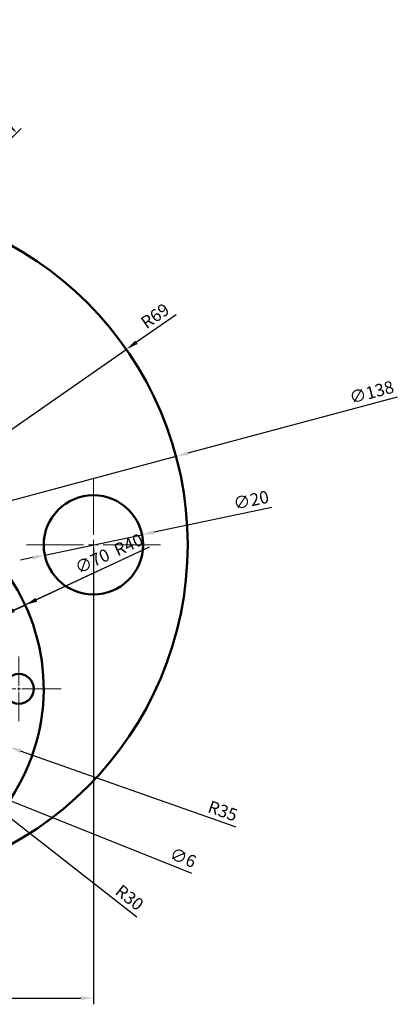
# Model space of a CAD drawing. Units: millimetres. Extents: x 3359 to 3569, y 1418 to 1617.
# Tile 2 of 2: x 3493 to 3569, y 1418 to 1617. Entities that reach past the tile are written whole.
import ezdxf

# ---------------------------------------------------------------- set-up
doc = ezdxf.new("R2010")
doc.units = ezdxf.units.MM
doc.linetypes.add('CENTER2', pattern=[28.575, 19.05, -3.175, 3.175, -3.175])
for name, color, linetype, lineweight in [('M-CNTR', 4, 'CENTER2', 18), ('M-CONS', 8, 'Continuous', 13), ('M-DIMS', 2, 'Continuous', 25), ('M-OUTL', 7, 'Continuous', 50)]:
    doc.layers.add(name, color=color, linetype=linetype, lineweight=lineweight)
doc.styles.get("Standard").update_dxf_attribs({"font": 'arial.ttf'})
doc.dimstyles.new('ISO-25', dxfattribs={"dimtxt": 2.5, "dimasz": 2.5, "dimexe": 1.25, "dimexo": 0.625, "dimtad": 1, "dimtxsty": 'Standard', "dimcen": 2.5, "dimadec": 0, "dimazin": 0, "dimtfac": 1, "dimtmove": 0, "dimatfit": 3, "dimfxl": 1, "dimarcsym": 0})

# ---------------------------------------------------------------- blocks, each defined once
blk = doc.blocks.new('*D1')
at = {"layer": 'Defpoints', "color": 0, "transparency": 16777216}
for p in [(3408.07, 1510.78), (3508.07, 1510.78), (3508.07, 1419.42)]:
    blk.add_point(p, dxfattribs=at)
at = {"layer": 'M-DIMS', "color": 0, "lineweight": -2, "transparency": 16777216}
for p, q in [((3408.07, 1510.16), (3408.07, 1418.17)), ((3508.07, 1510.16), (3508.07, 1418.17)), ((3410.57, 1419.42), (3505.57, 1419.42))]:
    blk.add_line(p, q, dxfattribs=at)
at = {"layer": 'M-DIMS', "color": 0, "transparency": 16777216}
for points in [[(3410.57, 1419.84), (3410.57, 1419), (3408.07, 1419.42)], [(3505.57, 1419.84), (3505.57, 1419), (3508.07, 1419.42)]]:
    blk.add_solid(points, dxfattribs=at)
at = {"layer": 'M-DIMS', "color": 0, "transparency": 16777216, "insert": (3458.07, 1421.32), "char_height": 2.5, "attachment_point": 5}
blk.add_mtext('100', dxfattribs=at)
blk = doc.blocks.new('*D9')
at = {"layer": 'Defpoints', "color": 0, "transparency": 16777216}
for p in [(3458.07, 1481.76), (3481.68, 1463.25)]:
    blk.add_point(p, dxfattribs=at)
at = {"layer": 'M-DIMS', "color": 0, "lineweight": -2, "transparency": 16777216}
for p, q in [((3458.07, 1481.76), (3481.68, 1463.25)), ((3516.82, 1435.71), (3483.65, 1461.71))]:
    blk.add_line(p, q, dxfattribs=at)
blk.add_arc((3458.07, 1481.76), 30, 316.7877, 324.2979, dxfattribs=at)
at = {"layer": 'M-DIMS', "color": 0, "transparency": 16777216}
blk.add_solid([(3483.91, 1462.04), (3483.39, 1461.38), (3481.68, 1463.25)], dxfattribs=at)
at = {"layer": 'M-DIMS', "color": 0, "transparency": 16777216, "insert": (3515.16, 1439.43), "char_height": 2.5, "attachment_point": 5, "rotation": 321.9105}
blk.add_mtext('R30', dxfattribs=at)
blk = doc.blocks.new('*D10')
at = {"layer": 'Defpoints', "color": 0, "transparency": 16777216}
for p in [(3458.07, 1481.76), (3491.06, 1470.06)]:
    blk.add_point(p, dxfattribs=at)
at = {"layer": 'M-DIMS', "color": 0, "lineweight": -2, "transparency": 16777216}
for p, q in [((3458.07, 1481.76), (3491.06, 1470.06)), ((3536.81, 1453.85), (3493.42, 1469.23))]:
    blk.add_line(p, q, dxfattribs=at)
at = {"layer": 'M-DIMS', "color": 0, "transparency": 16777216}
blk.add_solid([(3493.55, 1469.62), (3493.28, 1468.84), (3491.06, 1470.06)], dxfattribs=at)
at = {"layer": 'M-DIMS', "color": 0, "transparency": 16777216, "insert": (3534.03, 1456.85), "char_height": 2.5, "attachment_point": 5, "rotation": 340.485}
blk.add_mtext('R35', dxfattribs=at)
blk = doc.blocks.new('*D12')
at = {"layer": 'Defpoints', "color": 0, "transparency": 16777216}
for p in [(3514.7, 1550.2), (3458.07, 1510.78)]:
    blk.add_point(p, dxfattribs=at)
at = {"layer": 'M-DIMS', "color": 0, "lineweight": -2, "transparency": 16777216}
for p, q in [((3524.74, 1557.19), (3516.75, 1551.63)), ((3458.07, 1510.78), (3514.7, 1550.2))]:
    blk.add_line(p, q, dxfattribs=at)
at = {"layer": 'M-DIMS', "color": 0, "transparency": 16777216}
blk.add_solid([(3516.51, 1551.97), (3516.99, 1551.29), (3514.7, 1550.2)], dxfattribs=at)
at = {"layer": 'M-DIMS', "color": 0, "transparency": 16777216, "insert": (3520.68, 1556.69), "char_height": 2.5, "attachment_point": 5, "rotation": 34.8424}
blk.add_mtext('R69', dxfattribs=at)
blk = doc.blocks.new('*D17')
at = {"layer": 'Defpoints', "color": 0, "transparency": 16777216}
for p in [(3448.57, 1612.1), (3468.37, 1569.56), (3436.25, 1549.76), (3448.57, 1549.76), (3448.57, 1549.76)]:
    blk.add_point(p, dxfattribs=at)
at = {"layer": 'M-DIMS', "color": 0, "lineweight": -2, "transparency": 16777216}
for p, q in [((3468.81, 1570), (3493.54, 1594.73)), ((3435.62, 1549.76), (3384.97, 1549.76))]:
    blk.add_line(p, q, dxfattribs=at)
blk.add_arc((3448.57, 1549.76), 62.35, 47.2976, 177.7024, dxfattribs=at)
at = {"layer": 'M-DIMS', "color": 0, "transparency": 16777216}
for points in [[(3491.14, 1595.87), (3490.56, 1595.27), (3492.65, 1593.84)], [(3386.69, 1552.25), (3385.86, 1552.26), (3386.22, 1549.76)]]:
    blk.add_solid(points, dxfattribs=at)
at = {"layer": 'M-DIMS', "color": 0, "transparency": 16777216, "insert": (3423.98, 1609.11), "char_height": 2.5, "attachment_point": 5, "rotation": 22.5}
blk.add_mtext('135°', dxfattribs=at)
blk = doc.blocks.new('*D18')
at = {"layer": 'Defpoints', "color": 0, "transparency": 16777216}
for p in [(3483.6, 1462.3), (3489.17, 1460.07)]:
    blk.add_point(p, dxfattribs=at)
at = {"layer": 'M-DIMS', "color": 0, "lineweight": -2, "transparency": 16777216}
for p, q in [((3481.28, 1463.23), (3478.96, 1464.16)), ((3483.6, 1462.3), (3489.17, 1460.07)), ((3527.89, 1444.57), (3491.49, 1459.14))]:
    blk.add_line(p, q, dxfattribs=at)
at = {"layer": 'M-DIMS', "color": 0, "transparency": 16777216}
for points in [[(3481.43, 1463.61), (3481.12, 1462.84), (3483.6, 1462.3)], [(3491.65, 1459.53), (3491.34, 1458.75), (3489.17, 1460.07)]]:
    blk.add_solid(points, dxfattribs=at)
at = {"layer": 'M-DIMS', "color": 0, "transparency": 16777216, "insert": (3526.02, 1447.44), "char_height": 2.5, "attachment_point": 5, "rotation": 338.1832}
blk.add_mtext('∅6', dxfattribs=at)
blk = doc.blocks.new('*D19')
at = {"layer": 'Defpoints', "color": 0, "transparency": 16777216}
for p in [(3517.86, 1512.84), (3498.28, 1508.72)]:
    blk.add_point(p, dxfattribs=at)
at = {"layer": 'M-DIMS', "color": 0, "lineweight": -2, "transparency": 16777216}
for p, q in [((3544.01, 1518.35), (3520.3, 1513.36)), ((3498.28, 1508.72), (3517.86, 1512.84)), ((3495.84, 1508.21), (3493.39, 1507.69))]:
    blk.add_line(p, q, dxfattribs=at)
at = {"layer": 'M-DIMS', "color": 0, "transparency": 16777216}
for points in [[(3520.22, 1513.76), (3520.39, 1512.95), (3517.86, 1512.84)], [(3495.75, 1508.62), (3495.92, 1507.8), (3498.28, 1508.72)]]:
    blk.add_solid(points, dxfattribs=at)
at = {"layer": 'M-DIMS', "color": 0, "transparency": 16777216, "insert": (3539.91, 1519.5), "char_height": 2.5, "attachment_point": 5, "rotation": 11.8844}
blk.add_mtext('∅20', dxfattribs=at)
blk = doc.blocks.new('*U21')
at = {"layer": 'M-CNTR', "color": 0, "transparency": 16777216}
for p, q in [((0, 2), (0, 13.5)), ((-13.5, 0), (-2, 0)), ((2, 0), (13.5, 0)), ((0, -13.5), (0, -2))]:
    blk.add_line(p, q, dxfattribs=at)
at = {"layer": 'M-CNTR', "color": 0, "linetype": 'Continuous', "transparency": 16777216}
for p, q in [((-1, 0), (1, 0)), ((0, -1), (0, 1))]:
    blk.add_line(p, q, dxfattribs=at)
blk = doc.blocks.new('*U23')
at = {"layer": 'M-CNTR', "color": 0, "transparency": 16777216}
for p, q in [((0, 8), (0, 43.5)), ((-43.5, 0), (-8, 0)), ((8, 0), (43.5, 0)), ((0, -43.5), (0, -8))]:
    blk.add_line(p, q, dxfattribs=at)
at = {"layer": 'M-CNTR', "color": 0, "linetype": 'Continuous', "transparency": 16777216}
for p, q in [((0, -4), (0, 4)), ((-4, 0), (4, 0))]:
    blk.add_line(p, q, dxfattribs=at)
blk = doc.blocks.new('*U27')
at = {"layer": 'M-CNTR', "color": 0, "transparency": 16777216}
for p, q in [((0, 0.6), (0, 6.5)), ((-6.5, 0), (-0.6, 0)), ((0.6, 0), (6.5, 0)), ((0, -6.5), (0, -0.6))]:
    blk.add_line(p, q, dxfattribs=at)
at = {"layer": 'M-CNTR', "color": 0, "linetype": 'Continuous', "transparency": 16777216}
for p, q in [((-0.3, 0), (0.3, 0)), ((0, -0.3), (0, 0.3))]:
    blk.add_line(p, q, dxfattribs=at)
blk = doc.blocks.new('BOLT-HOLE-D6')
blk.add_circle((0, 0), 3)
blk = doc.blocks.new('MOUNT-HOLE-D20')
blk.add_circle((0, 0), 10)
blk = doc.blocks.new('*D38')
at = {"layer": 'Defpoints', "color": 0, "transparency": 16777216}
for p in [(3524.72, 1528.64), (3391.42, 1492.92)]:
    blk.add_point(p, dxfattribs=at)
at = {"layer": 'M-DIMS', "color": 0, "lineweight": -2, "transparency": 16777216}
for p, q in [((3569.29, 1540.59), (3527.13, 1529.29)), ((3391.42, 1492.92), (3524.72, 1528.64)), ((3389.01, 1492.28), (3386.59, 1491.63))]:
    blk.add_line(p, q, dxfattribs=at)
at = {"layer": 'M-DIMS', "color": 0, "transparency": 16777216}
for points in [[(3527.03, 1529.69), (3527.24, 1528.89), (3524.72, 1528.64)], [(3388.9, 1492.68), (3389.11, 1491.87), (3391.42, 1492.92)]]:
    blk.add_solid(points, dxfattribs=at)
at = {"layer": 'M-DIMS', "color": 0, "transparency": 16777216, "insert": (3564.2, 1541.26), "char_height": 2.5, "attachment_point": 5, "rotation": 15.0008}
blk.add_mtext('∅138', dxfattribs=at)
blk = doc.blocks.new('*D39')
at = {"layer": 'Defpoints', "color": 0, "transparency": 16777216}
for p in [(3494.32, 1498.66), (3458.07, 1481.76)]:
    blk.add_point(p, dxfattribs=at)
at = {"layer": 'M-DIMS', "color": 0, "lineweight": -2, "transparency": 16777216}
for p, q in [((3519.34, 1510.33), (3496.59, 1499.72)), ((3458.07, 1481.76), (3494.32, 1498.66))]:
    blk.add_line(p, q, dxfattribs=at)
at = {"layer": 'M-DIMS', "color": 0, "transparency": 16777216}
blk.add_solid([(3496.41, 1500.1), (3496.76, 1499.34), (3494.32, 1498.66)], dxfattribs=at)
at = {"layer": 'M-DIMS', "color": 0, "transparency": 16777216, "insert": (3515.27, 1510.53), "char_height": 2.5, "attachment_point": 5, "rotation": 25.0008}
blk.add_mtext('R40', dxfattribs=at)
blk = doc.blocks.new('*D40')
at = {"layer": 'Defpoints', "color": 0, "transparency": 16777216}
for p in [(3489.79, 1496.55), (3426.35, 1466.96)]:
    blk.add_point(p, dxfattribs=at)
at = {"layer": 'M-DIMS', "color": 0, "lineweight": -2, "transparency": 16777216}
for p, q in [((3512.24, 1507.02), (3492.06, 1497.61)), ((3426.35, 1466.96), (3489.79, 1496.55)), ((3424.08, 1465.91), (3421.82, 1464.85))]:
    blk.add_line(p, q, dxfattribs=at)
at = {"layer": 'M-DIMS', "color": 0, "transparency": 16777216}
for points in [[(3491.88, 1497.98), (3492.23, 1497.23), (3489.79, 1496.55)], [(3423.91, 1466.29), (3424.26, 1465.53), (3426.35, 1466.96)]]:
    blk.add_solid(points, dxfattribs=at)
at = {"layer": 'M-DIMS', "color": 0, "transparency": 16777216, "insert": (3507.99, 1507.21), "char_height": 2.5, "attachment_point": 5, "rotation": 25.0014}
blk.add_mtext('∅70', dxfattribs=at)

msp = doc.modelspace()

# ---------------------------------------------------------------- linework, layer by layer
at = {"layer": 'M-CONS'}
msp.add_line((3508.0696, 1510.7826), (3508.0696, 1506.0048), dxfattribs=at)
at = {"layer": 'M-OUTL'}
msp.add_circle((3458.0696, 1510.7826), 69, dxfattribs=at)
msp.add_arc((3458.0696, 1481.7566), 40, 130.541602, 49.458398, dxfattribs=at)

# ---------------------------------------------------------------- block references
at = {"layer": 'M-CNTR'}
for name, p in [('*U23', (3458.0696, 1481.7566)), ('*U21', (3508.0696, 1510.7826)), ('*U27', (3493.0696, 1481.7566))]:
    msp.add_blockref(name, p, dxfattribs=at)
at = {"layer": 'M-OUTL'}
for name, p in [('MOUNT-HOLE-D20', (3508.0696, 1510.7826)), ('BOLT-HOLE-D6', (3493.0696, 1481.7566))]:
    msp.add_blockref(name, p, dxfattribs=at)

# ---------------------------------------------------------------- dimensions: what is measured, and where the dimension line sits
at = {"layer": 'M-DIMS'}
dim = msp.add_angular_dim_2l(base=(3448.5696, 1612.1025), line1=((3448.5696, 1549.7566), (3468.3686, 1569.5556)), line2=((3448.5696, 1549.7566), (3436.2452, 1549.7566)), dimstyle='ISO-25', override={"dimclrd": 0, "dimclre": 0, "dimclrt": 0}, dxfattribs=at)
dim.commit()
dim.dimension.update_dxf_attribs({"geometry": '*D17', "text_midpoint": (3423.9829, 1609.1142)})
dim = msp.add_radius_dim(center=(3458.0696, 1510.7826), mpoint=(3514.6997, 1550.2038), dimstyle='ISO-25', override={"dimclrd": 0, "dimclre": 0, "dimclrt": 0}, dxfattribs=at)
dim.commit()
dim.dimension.update_dxf_attribs({"geometry": '*D12', "text_midpoint": (3520.6835, 1556.6859)})
for p1, p2, override, picture, middle in [((3391.4209, 1492.9231), (3524.7182, 1528.6421), {"dimdec": 0, "dimlfac": 1, "dimrnd": 0, "dimzin": 0, "dimdsep": 46, "dimlunit": 2}, '*D38', (3564.7074, 1539.3577)), ((3498.2839, 1508.7232), (3517.8552, 1512.842), {"dimclrd": 0, "dimclre": 0, "dimclrt": 0}, '*D19', (3540.3202, 1517.5697)), ((3426.3492, 1466.9642), (3489.79, 1496.549), {"dimdec": 0, "dimlfac": 1, "dimrnd": 0, "dimzin": 0, "dimdsep": 46, "dimlunit": 2}, '*D40', (3508.8222, 1505.4244)), ((3483.6, 1462.299), (3489.1703, 1460.0692), {"dimclrd": 0, "dimclre": 0, "dimclrt": 0}, '*D18', (3525.2868, 1445.6113))]:
    dim = msp.add_diameter_dim_2p(p1=p1, p2=p2, dimstyle='ISO-25', override=override, dxfattribs=at)
    dim.commit()
    dim.dimension.update_dxf_attribs({"geometry": picture, "text_midpoint": middle, "dimtype": 163})
for mpoint, override, picture, middle in [((3494.3216, 1498.6618), {"dimdec": 0, "dimlfac": 1, "dimrnd": 0, "dimzin": 0, "dimdsep": 46, "dimlunit": 2}, '*D39', (3516.0729, 1508.805)), ((3481.681, 1463.2498), {"dimclrd": 0, "dimclre": 0, "dimclrt": 0}, '*D9', (3513.9826, 1437.9318)), ((3491.059, 1470.0647), {"dimclrd": 0, "dimclre": 0, "dimclrt": 0}, '*D10', (3533.3951, 1455.0603))]:
    dim = msp.add_radius_dim(center=(3458.0696, 1481.7566), mpoint=mpoint, dimstyle='ISO-25', override=override, dxfattribs=at)
    dim.commit()
    dim.dimension.update_dxf_attribs({"geometry": picture, "text_midpoint": middle, "dimtype": 164})
dim = msp.add_linear_dim(base=(3508.0696, 1419.4191), p1=(3408.0696, 1510.7826), p2=(3508.0696, 1510.7826), dimstyle='ISO-25', override={"dimclrd": 0, "dimclre": 0, "dimclrt": 0}, dxfattribs=at)
dim.commit()
dim.dimension.update_dxf_attribs({"geometry": '*D1', "text_midpoint": (3458.0696, 1421.3206)})

doc.saveas('drawing.dxf')
